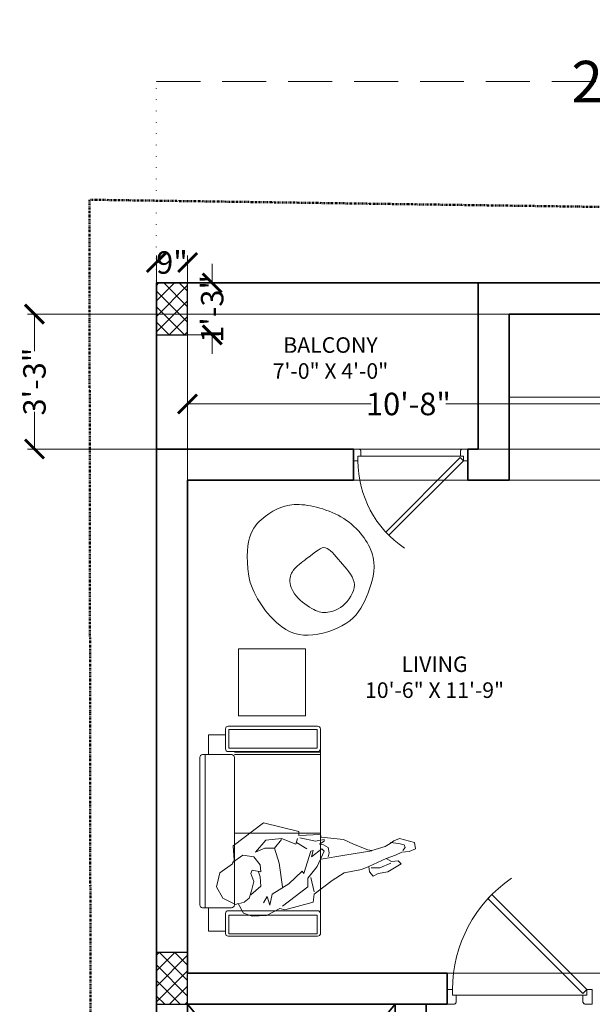
# Model space of a CAD drawing. Units: inches. Extents: x -16911 to -9621, y -48626 to -46270.
# Tile 13 of 20: x -12101 to -11935, y -46595 to -46311. Entities that reach past the tile are written whole.
import ezdxf

# ---------------------------------------------------------------- set-up
doc = ezdxf.new("R2010")
doc.units = ezdxf.units.IN
for name, pattern in [('DASHDOT', [1, 0.5, -0.25, 0, -0.25]), ('DASHED', [19.05, 12.7, -6.35]), ('DOT2', [3.175, 0, -3.175])]:
    doc.linetypes.add(name, pattern=pattern)
for name, color, linetype, lineweight in [('A-ANNO-DIMS', 2, 'Continuous', 13), ('A-AREA-IDEN', 3, 'Continuous', 18), ('A-DOOR', 4, 'Continuous', 18), ('A-FURN', 8, 'Continuous', 13), ('A-WALL', 7, 'Continuous', 35), ('C-PROP', 6, 'DASHDOT', 50), ('column', 12, 'Continuous', 30), ('DOOR', 143, 'Continuous', 9), ('EXT BEAM', 132, 'Continuous', 13), ('furniture', 35, 'Continuous', 15), ('Man', 8, 'Continuous', 5), ('S-BEAM', 132, 'Continuous', 25), ('S-COLS', 1, 'Continuous', 30)]:
    doc.layers.add(name, color=color, linetype=linetype, lineweight=lineweight)
doc.styles.add('style3', font='times.ttf')
doc.styles.add('style9', font='swisscl.ttf', dxfattribs={"height": 12})
doc.dimstyles.new('Dim9', dxfattribs={"dimtxt": 10, "dimasz": 0.199219, "dimexe": 1, "dimexo": 0.5, "dimgap": 1, "dimtad": 0, "dimdec": 1, "dimzin": 0, "dimdsep": 46, "dimlunit": 4, "dimtxsty": 'style9', "dimblk": 'ARCHTICK', "dimcen": 0.09, "dimclrd": 256, "dimclrt": 256, "dimadec": 0, "dimazin": 0, "dimtfac": 1, "dimtdec": 1, "dimtix": 1, "dimtofl": 0, "dimtmove": 1, "dimatfit": 3, "dimfxl": 9, "dimtolj": 1, "dimtzin": 0, "dimlwd": -1, "dimarcsym": 0})
doc.dimstyles.new('S.S.S', dxfattribs={"dimtxt": 6.5, "dimasz": 5.5, "dimexe": 2, "dimexo": 0, "dimgap": 0.09, "dimtad": 0, "dimdec": 1, "dimzin": 3, "dimdsep": 46, "dimlunit": 4, "dimtxsty": 'style3', "dimblk": 'ARCHTICK', "dimcen": 2.5, "dimclrd": 252, "dimclre": 256, "dimclrt": 7, "dimadec": 0, "dimazin": 0, "dimtfac": 1, "dimtdec": 1, "dimtix": 1, "dimtofl": 0, "dimtmove": 0, "dimatfit": 3, "dimfxl": 2, "dimtolj": 1, "dimtzin": 0, "dimlwd": 13, "dimlwe": 15, "dimarcsym": 0})

# ---------------------------------------------------------------- blocks, each defined once
blk = doc.blocks.new('Bipman02')
blk.add_lwpolyline([(0.5871, -0.067), (0.6175, -0.0496), (0.6523, -0.0539), (0.6697, -0.0376), (0.5958, 0.0069), (0.5437, 0.0156), (0.5164, 0.0297), (0.4959, 0.0069), (0.4915, -0.0235), (0.4524, -0.0061), (0.3568, 0.0113), (0.2917, 0.0548), (0.1917, 0.1287), (0.1874, 0.1722), (0.031, 0.2156), (0.0049, 0.2069), (-0.0689, 0.2461), (-0.1471, 0.2504), (-0.1949, 0.233), (-0.2253, 0.1808), (-0.2384, 0.1852), (-0.3079, 0.1504), (-0.3426, 0.0895), (-0.3253, 0.0113), (-0.2558, -0.0365), (-0.2471, -0.0583), (-0.2514, -0.1365), (-0.0863, -0.2626), (0.1092, -0.2148), (0.1092, -0.193), (0.2265, -0.1974), (0.2308, -0.1844), (0.3525, -0.1713), (0.409, -0.1452), (0.4872, -0.1148), (0.5089, -0.1104), (0.5828, -0.1322), (0.6088, -0.1496), (0.6295, -0.1636), (0.661, -0.1757), (0.7435, -0.1539), (0.7478, -0.1191), (0.7143, -0.1051), (0.674, -0.1017), (0.6392, -0.0844)], close=True)
for points in [[(-0.2558, -0.0452), (-0.1993, -0.0844), (-0.1385, -0.0757), (-0.1037, -0.0322), (-0.0994, 0.0069), (-0.1471, -0.0018), (-0.1558, 0.0156), (-0.1385, 0.0591), (-0.1515, 0.1113), (-0.1645, 0.1504), (-0.1906, 0.1722), (-0.2167, 0.1808)], [(-0.0863, 0.1765), (-0.0646, 0.1417), (-0.0516, 0.1895), (-0.0385, 0.1287), (0.0527, 0.0722), (0.1266, 0.0026), (0.1353, 0.0156), (0.1744, -0.1061), (0.1874, -0.1104), (0.1787, -0.0757), (0.2352, -0.1191), (0.2482, -0.1061), (0.2091, -0.0235), (0.157, 0.0417), (0.157, 0.0895), (0.018, 0.1939)], [(-0.1558, 0.133), (-0.0994, 0.0852), (-0.1037, 0.033), (-0.1124, 0.0069)], [(0.1917, 0.1156), (0.1744, 0.0374)], [(0.018, 0.0895), (0.0006, -0.0409), (-0.0255, -0.1235), (-0.0776, -0.1235), (-0.1298, -0.1017), (-0.0733, -0.167), (0.0136, -0.1757), (0.0918, -0.1452), (0.1005, -0.1757)], [(0.4915, -0.0235), (0.5871, -0.067)], [(0.5045, -0.0148), (0.5523, -0.0148), (0.6132, -0.0409)], [(0.2699, -0.0757), (0.2743, -0.0974), (0.2699, -0.1278), (0.2439, -0.1409), (0.2222, -0.1452), (0.2482, -0.1626), (0.2482, -0.1713), (0.2004, -0.1626), (0.1135, -0.18)], [(0.2308, -0.0626), (0.3612, -0.0844), (0.5089, -0.1095)], [(-0.0255, -0.1235), (0.0136, -0.1713)], [(0.0962, -0.1539), (0.1526, -0.1191)], [(0.6783, -0.1104), (0.6914, -0.1278), (0.687, -0.1409), (0.6566, -0.1496), (0.6088, -0.1539)]]:
    blk.add_lwpolyline(points)
blk = doc.blocks.new('erertety')
at = {"layer": 'furniture', "ltscale": 0.2}
for p, q in [((-17662.13, -45230.66), (-17662.13, -45176.69)), ((-17693.83, -45223.2), (-17693.83, -45184.43)), ((-17685.49, -45183.68), (-17693.08, -45183.68)), ((-17684.74, -45223.2), (-17684.74, -45184.43)), ((-17684.74, -45203.31), (-17662.13, -45203.31)), ((-17685.49, -45223.95), (-17693.08, -45223.95)), ((-17691.58, -45223.95), (-17691.58, -45229.1)), ((-17684.74, -45223.99), (-17662.13, -45223.99)), ((-17684.74, -45224.55), (-17662.13, -45224.55)), ((-17684.74, -45224.55), (-17662.13, -45224.55)), ((-17691.58, -45229.1), (-17687.09, -45229.1))]:
    blk.add_line(p, q, dxfattribs=at)
for points in [[(-17662.13, -45182.17), (-17662.13, -45176.97, 0.414214), (-17662.87, -45176.22), (-17686.34, -45176.22, 0.414214), (-17687.09, -45176.97), (-17687.09, -45182.17, 0.414214), (-17686.34, -45182.91), (-17662.87, -45182.91, 0.414214)], [(-17662.13, -45225.47), (-17662.13, -45230.66, -0.414214), (-17662.87, -45231.41), (-17686.34, -45231.41, -0.414214), (-17687.09, -45230.66), (-17687.09, -45225.47, -0.414214), (-17686.34, -45224.72), (-17662.87, -45224.72, -0.414214)]]:
    blk.add_lwpolyline(points, format="xyb", close=True, dxfattribs=at)
for points in [[(-17663.01, -45181.75), (-17663.01, -45176.82), (-17686.21, -45176.82), (-17686.21, -45181.75)], [(-17692.4, -45183.68), (-17692.4, -45223.95), (-17692.4, -45223.95), (-17692.4, -45183.68)], [(-17663.01, -45225.6), (-17663.01, -45230.53), (-17686.21, -45230.53), (-17686.21, -45225.6)]]:
    blk.add_lwpolyline(points, close=True, dxfattribs=at)
blk.add_lwpolyline([(-17687.09, -45177.54), (-17691.58, -45177.54), (-17691.58, -45183.68)], dxfattribs=at)
for centre, start, end in [((-17693.08, -45184.43), 90, 180), ((-17685.49, -45184.43), 0, 90), ((-17693.08, -45223.2), 180, 270), ((-17685.49, -45223.2), 270, 0)]:
    blk.add_arc(centre, 0.748, start, end, dxfattribs=at)
at = {"layer": 'furniture', "ltscale": 0.2, "xscale": 47.90818138957024, "yscale": 47.90818138957024, "zscale": 47.90818138957024}
blk.add_blockref('Bipman02', (-17673, -45193.44, 0), dxfattribs=at)
blk = doc.blocks.new('rthrty')
at = {"layer": 'furniture'}
blk.add_open_spline([(-17650.3, -45154.53), (-17651.97, -45142.9), (-17645.3, -45136.31), (-17637.11, -45132.37), (-17620.71, -45137.17), (-17612.47, -45149.45), (-17615.73, -45159.71), (-17619.67, -45168.02), (-17632.28, -45172.65), (-17641.84, -45170.43), (-17649.5, -45159.42), (-17650.3, -45154.53)], degree=3, dxfattribs=at)
at = {"layer": 'Man'}
blk.add_open_spline([(-17632.99, -45149.02), (-17629.89, -45146.6), (-17628, -45145.12), (-17623.29, -45151.15), (-17618.06, -45156.77), (-17623.15, -45164.08), (-17628.28, -45165.32), (-17631.61, -45164.6), (-17638.01, -45159.61), (-17638.81, -45154.69), (-17636.9, -45151.81), (-17632.99, -45149.02), (-17632.99, -45149.02)], degree=3, dxfattribs=at)
blk = doc.blocks.new('A$C1C9D3E54')
at = {"layer": 'DOOR'}
blk.add_line((18676.53, 5780.72), (18710.53, 5780.72), dxfattribs=at)
blk.add_lwpolyline([(18685.01, 5806.62), (18710.47, 5781.16), (18711.53, 5782.22), (18686.07, 5807.68), (18685.01, 5806.62)], dxfattribs=at)
blk.add_lwpolyline([(18674.03, 5778.22), (18676.03, 5778.22), (18674.03, 5778.22), (18674.03, 5782.22), (18675.53, 5782.22), (18675.53, 5780.72), (18676.53, 5780.72), (18676.53, 5778.72), (18676.41, 5778.72), (18676.41, 5778.6, -0.414214), (18676.16, 5778.35), (18676.03, 5778.35), (18676.03, 5778.22)], format="xyb", dxfattribs=at)
blk.add_lwpolyline([(18713.03, 5782.22), (18711.53, 5782.22), (18711.53, 5780.72), (18710.53, 5780.72), (18710.53, 5778.72), (18710.66, 5778.72), (18710.66, 5778.6, 0.414214), (18710.91, 5778.35), (18711.03, 5778.35), (18711.03, 5778.22), (18713.03, 5778.22), (18711.03, 5778.22), (18713.03, 5778.22), (18713.03, 5782.22)], format="xyb", close=True, dxfattribs=at)
blk.add_arc((18711.53, 5782.22), 36, 124.0336, 180, dxfattribs=at)
blk = doc.blocks.new('COLUMNS')
at = {"layer": 'column'}
h = blk.add_hatch(dxfattribs=at)
h.set_pattern_fill('ANSI37', color=256, angle=-720)
h.set_pattern_definition([(45, (21703.4588, -104481.6704), (-2.24506403, 2.24506403), []), (135, (21703.4588, -104481.6704), (-2.24506403, -2.24506403), [])])
h.paths.add_polyline_path([(-12061.47, -46401.86), (-12052.47, -46401.86), (-12052.47, -46386.86), (-12061.47, -46386.86)])
h = blk.add_hatch(dxfattribs=at)
h.set_pattern_fill('ANSI37', color=256, angle=-900)
h.set_pattern_definition([(225, (-45817.4075, 11499.4594), (2.24506403, -2.24506403), []), (315, (-45817.4075, 11499.4594), (2.24506403, 2.24506403), [])])
h.paths.add_polyline_path([(-12052.47, -46580.36), (-12061.47, -46580.36), (-12061.47, -46595.36), (-12052.47, -46595.36)])
at = {"layer": 'column', "ltscale": 0.05}
for points in [[(-12052.47, -46386.86), (-12061.47, -46386.86), (-12061.47, -46401.86), (-12052.47, -46401.86)], [(-12061.47, -46595.36), (-12052.47, -46595.36), (-12052.47, -46580.36), (-12061.47, -46580.36)]]:
    blk.add_lwpolyline(points, close=True, dxfattribs=at)
blk = doc.blocks.new('TYPICAL BEAMS G-2')
at = {"layer": 'EXT BEAM'}
for p, q in [((-12061.47, -47658.74), (-11738.92, -47658.74)), ((-12061.47, -48216.7), (-12061.47, -47658.74)), ((-12052.47, -47667.74), (-11924.72, -47667.74)), ((-12052.47, -47939.24), (-12052.47, -47667.74)), ((-12052.47, -47706.74), (-11924.72, -47706.74)), ((-12052.47, -47715.74), (-11924.72, -47715.74)), ((-12052.47, -47858.24), (-11924.72, -47858.24))]:
    blk.add_line(p, q, dxfattribs=at)
blk = doc.blocks.new('_ArchTick')
at = {"color": 0, "linetype": 'ByBlock', "const_width": 0.15}
blk.add_lwpolyline([(-0.5, -0.5), (0.5, 0.5)], dxfattribs=at)
blk = doc.blocks.new('*D44')
at = {"layer": 'A-ANNO-DIMS', "color": 0, "lineweight": 15, "transparency": 16777216}
for p, q in [((-12052.47, -46395.86), (-12098.73, -46395.86)), ((-12052.47, -46434.86), (-12098.73, -46434.86))]:
    blk.add_line(p, q, dxfattribs=at)
at = {"layer": 'A-ANNO-DIMS', "color": 0, "lineweight": 13, "transparency": 16777216}
for p, q in [((-12096.73, -46395.86), (-12096.73, -46406.56)), ((-12096.73, -46434.86), (-12096.73, -46424.15))]:
    blk.add_line(p, q, dxfattribs=at)
at = {"layer": 'Defpoints', "color": 0, "transparency": 16777216}
for p in [(-12052.47, -46395.86), (-12096.73, -46434.86), (-12052.47, -46434.86)]:
    blk.add_point(p, dxfattribs=at)
at = {"layer": 'A-ANNO-DIMS', "color": 0, "lineweight": 13, "transparency": 16777216, "xscale": 5.5, "yscale": 5.5, "zscale": 5.5}
for p, rotation in [((-12096.73, -46395.86), 90), ((-12096.73, -46434.86), 270)]:
    blk.add_blockref('_ArchTick', p, dxfattribs=dict(at, rotation=rotation))
at = {"layer": 'A-ANNO-DIMS', "color": 0, "transparency": 16777216, "insert": (-12096.73, -46415.36), "char_height": 6.5, "attachment_point": 5, "rotation": 90, "style": 'style3'}
blk.add_mtext('\\A1;3\'-3"', dxfattribs=at)
blk = doc.blocks.new('*D45')
at = {"layer": 'A-ANNO-DIMS', "color": 0, "lineweight": 15, "transparency": 16777216}
for p, q in [((-12052.47, -46434.86), (-12052.47, -46419.84)), ((-11924.72, -46434.86), (-11924.72, -46419.84))]:
    blk.add_line(p, q, dxfattribs=at)
at = {"layer": 'A-ANNO-DIMS', "color": 0, "lineweight": 13, "transparency": 16777216}
for p, q in [((-12052.47, -46421.84), (-11999.43, -46421.84)), ((-11924.72, -46421.84), (-11977.77, -46421.84))]:
    blk.add_line(p, q, dxfattribs=at)
at = {"layer": 'Defpoints', "color": 0, "transparency": 16777216}
for p in [(-11924.72, -46421.84), (-12052.47, -46434.86), (-11924.72, -46434.86)]:
    blk.add_point(p, dxfattribs=at)
at = {"layer": 'A-ANNO-DIMS', "color": 0, "lineweight": 13, "transparency": 16777216, "xscale": 5.5, "yscale": 5.5, "zscale": 5.5, "rotation": 180}
blk.add_blockref('_ArchTick', (-12052.47, -46421.84), dxfattribs=at)
at = {"layer": 'A-ANNO-DIMS', "color": 0, "lineweight": 13, "transparency": 16777216, "xscale": 5.5, "yscale": 5.5, "zscale": 5.5}
blk.add_blockref('_ArchTick', (-11924.72, -46421.84), dxfattribs=at)
at = {"layer": 'A-ANNO-DIMS', "color": 0, "transparency": 16777216, "insert": (-11988.6, -46421.84), "char_height": 6.5, "attachment_point": 5, "style": 'style3'}
blk.add_mtext('\\A1;10\'-8"', dxfattribs=at)
blk = doc.blocks.new('*D48')
at = {"layer": 'A-ANNO-DIMS', "color": 0, "lineweight": 15, "transparency": 16777216}
for p, q in [((-12061.47, -46386.86), (-12061.47, -46378.94)), ((-12052.47, -46386.86), (-12052.47, -46378.94))]:
    blk.add_line(p, q, dxfattribs=at)
at = {"layer": 'A-ANNO-DIMS', "color": 0, "lineweight": 13, "transparency": 16777216}
for p, q in [((-12061.47, -46380.94), (-12060.91, -46380.94)), ((-12052.47, -46380.94), (-12053.03, -46380.94))]:
    blk.add_line(p, q, dxfattribs=at)
at = {"layer": 'Defpoints', "color": 0, "transparency": 16777216}
for p in [(-12052.47, -46380.94), (-12061.47, -46386.86), (-12052.47, -46386.86)]:
    blk.add_point(p, dxfattribs=at)
at = {"layer": 'A-ANNO-DIMS', "color": 0, "lineweight": 13, "transparency": 16777216, "xscale": 5.5, "yscale": 5.5, "zscale": 5.5, "rotation": 180}
blk.add_blockref('_ArchTick', (-12061.47, -46380.94), dxfattribs=at)
at = {"layer": 'A-ANNO-DIMS', "color": 0, "lineweight": 13, "transparency": 16777216, "xscale": 5.5, "yscale": 5.5, "zscale": 5.5}
blk.add_blockref('_ArchTick', (-12052.47, -46380.94), dxfattribs=at)
at = {"layer": 'A-ANNO-DIMS', "color": 0, "transparency": 16777216, "insert": (-12056.97, -46380.94), "char_height": 6.5, "attachment_point": 5, "style": 'style3'}
blk.add_mtext('\\A1;9"', dxfattribs=at)
blk = doc.blocks.new('*D49')
at = {"layer": 'A-ANNO-DIMS', "color": 0, "lineweight": 13, "transparency": 16777216}
for p, q in [((-12045.35, -46386.86), (-12045.35, -46381.36)), ((-12045.35, -46401.86), (-12045.35, -46407.36))]:
    blk.add_line(p, q, dxfattribs=at)
at = {"layer": 'A-ANNO-DIMS', "color": 0, "lineweight": 15, "transparency": 16777216}
for p, q in [((-12052.47, -46386.86), (-12043.35, -46386.86)), ((-12052.47, -46401.86), (-12043.35, -46401.86))]:
    blk.add_line(p, q, dxfattribs=at)
at = {"layer": 'Defpoints', "color": 0, "transparency": 16777216}
for p in [(-12052.47, -46386.86), (-12052.47, -46401.86), (-12045.35, -46401.86)]:
    blk.add_point(p, dxfattribs=at)
at = {"layer": 'A-ANNO-DIMS', "color": 0, "lineweight": 13, "transparency": 16777216, "xscale": 5.5, "yscale": 5.5, "zscale": 5.5}
for p, rotation in [((-12045.35, -46386.86), 270), ((-12045.35, -46401.86), 90)]:
    blk.add_blockref('_ArchTick', p, dxfattribs=dict(at, rotation=rotation))
at = {"layer": 'A-ANNO-DIMS', "color": 0, "transparency": 16777216, "insert": (-12045.35, -46394.36), "char_height": 6.5, "attachment_point": 5, "rotation": 90, "style": 'style3'}
blk.add_mtext('\\A1;1\'-3"', dxfattribs=at)
blk = doc.blocks.new('*D114')
at = {"layer": 'A-ANNO-DIMS', "color": 0, "linetype": 'DOT2', "lineweight": -2, "transparency": 16777216}
for p, q in [((-12061.47, -46386.36), (-12061.47, -46327.66)), ((-11738.92, -46386.36), (-11738.92, -46327.66))]:
    blk.add_line(p, q, dxfattribs=at)
at = {"layer": 'A-ANNO-DIMS', "linetype": 'DASHED', "transparency": 16777216}
for p, q in [((-12061.47, -46328.66), (-11933.21, -46328.66)), ((-11738.92, -46328.66), (-11867.19, -46328.66))]:
    blk.add_line(p, q, dxfattribs=at)
at = {"layer": 'Defpoints', "color": 0, "transparency": 16777216}
for p in [(-11738.92, -46328.66), (-12061.47, -46386.86), (-11738.92, -46386.86)]:
    blk.add_point(p, dxfattribs=at)
at = {"layer": 'A-ANNO-DIMS', "transparency": 16777216, "xscale": 0.19921875, "yscale": 0.19921875, "zscale": 0.19921875, "rotation": 180}
blk.add_blockref('_ArchTick', (-12061.47, -46328.66), dxfattribs=at)
at = {"layer": 'A-ANNO-DIMS', "transparency": 16777216, "xscale": 0.19921875, "yscale": 0.19921875, "zscale": 0.19921875}
blk.add_blockref('_ArchTick', (-11738.92, -46328.66), dxfattribs=at)
at = {"layer": 'A-ANNO-DIMS', "transparency": 16777216, "insert": (-11900.2, -46328.66), "char_height": 12, "attachment_point": 5, "style": 'style9'}
blk.add_mtext('\\A1;26\'-10 1/2"', dxfattribs=at)

msp = doc.modelspace()

# ---------------------------------------------------------------- linework, layer by layer
at = {"layer": 'A-FURN', "ltscale": 0.2}
msp.add_line((-11795.925, -46419.855), (-11959.474, -46419.855), dxfattribs=at)
at = {"layer": 'A-FURN'}
msp.add_lwpolyline([(-12018.353, -46511.978), (-12037.713, -46511.978), (-12037.713, -46492.618), (-12018.353, -46492.618)], close=True, dxfattribs=at)
at = {"layer": 'A-WALL'}
for p, q in [((-12061.474, -46434.855), (-12061.474, -46386.855)), ((-11968.474, -46386.855), (-12061.474, -46386.855)), ((-11968.474, -46434.855), (-11968.474, -46386.855)), ((-11738.925, -46386.855), (-11968.474, -46386.855)), ((-11959.474, -46443.855), (-11959.474, -46395.855)), ((-11795.925, -46395.855), (-11959.474, -46395.855)), ((-12061.474, -46896.809), (-12061.474, -46434.855)), ((-12004.474, -46434.855), (-12061.474, -46434.855)), ((-12004.474, -46434.855), (-12004.474, -46443.855)), ((-11968.474, -46434.855), (-11971.474, -46434.855)), ((-11971.474, -46434.855), (-11971.474, -46443.855)), ((-12052.474, -46586.355), (-12052.474, -46443.855)), ((-12004.474, -46443.855), (-12052.474, -46443.855)), ((-11959.474, -46443.855), (-11971.474, -46443.855)), ((-11977.474, -46586.355), (-12052.474, -46586.355)), ((-11977.474, -46595.355), (-11977.474, -46586.355)), ((-12052.474, -46667.355), (-12052.474, -46595.355)), ((-11977.474, -46595.355), (-12052.474, -46595.355)), ((-12052.474, -46595.355), (-11992.474, -46667.355)), ((-12052.474, -46667.355), (-11992.474, -46595.355)), ((-11992.474, -46667.355), (-11992.474, -46595.355)), ((-11983.474, -46667.355), (-11983.474, -46595.355))]:
    msp.add_line(p, q, dxfattribs=at)
at = {"layer": 'C-PROP'}
msp.add_lwpolyline([(-12080.474, -46962.809), (-11720.293, -46969.035), (-11719.732, -46940.446), (-11720.395, -46855.606), (-11721.561, -46609.511), (-11721.175, -46367.855), (-12080.838, -46362.811), (-12080.3, -46762.955)], close=True, dxfattribs=at)

# ---------------------------------------------------------------- block references
at = {"layer": 'A-DOOR', "xscale": -0.8461538461538624, "yscale": 0.8461538461538624, "zscale": 0.8461538461538624, "rotation": 180}
msp.add_blockref('A$C1C9D3E54', (-27805.577, -41545.589), dxfattribs=at)
at = {"layer": 'A-DOOR', "xscale": 1.076923076922859, "yscale": 1.076923076922859, "zscale": 1.076923076922859}
msp.add_blockref('A$C1C9D3E54', (-32087.969, -52818.058), dxfattribs=at)
at = {"layer": 'A-FURN'}
msp.add_blockref('rthrty', (5615.537, -1317.075), dxfattribs=at)
at = {"layer": 'A-FURN', "xscale": -1.1, "yscale": 1.1, "zscale": 1.1, "rotation": 180}
msp.add_blockref('erertety', (7414.285, -96269.509, 0), dxfattribs=at)
at = {"layer": 'S-BEAM'}
msp.add_blockref('TYPICAL BEAMS G-2', (0, 1271.886), dxfattribs=at)
at = {"layer": 'S-COLS'}
msp.add_blockref('COLUMNS', (0, 0), dxfattribs=at)

# ---------------------------------------------------------------- texts
at = {"layer": 'A-AREA-IDEN', "ltscale": 10, "char_height": 4.5, "width": 42.823, "attachment_point": 1, "style": 'style9'}
for s, insert in [('\\A1;\\pxqc;{\\fCentury Gothic|b0|i0|c0|p34;BALCONY\\P7\'-0" X 4\'-0"}', (-12032.568, -46402.553)), ('\\A1;\\pxqc;{\\fCentury Gothic|b0|i0|c0|p34;LIVING\\P10\'-6" X 11\'-9"}', (-12002.486, -46494.801))]:
    msp.add_mtext(s, dxfattribs=dict(at, insert=insert))

# ---------------------------------------------------------------- dimensions: what is measured, and where the dimension line sits
at = {"layer": 'A-ANNO-DIMS'}
for base, p1, p2, dimstyle, override, picture, middle in [((-11738.925, -46328.661), (-12061.474, -46386.855), (-11738.925, -46386.855), 'Dim9', {"dimdec": 1, "dimlfac": 1, "dimrnd": 0, "dimzin": 1, "dimdsep": 46, "dimlunit": 4, "dimfrac": 2}, '*D114', (-11900.199, -46328.661)), ((-12052.474, -46380.945), (-12061.474, -46386.855), (-12052.474, -46386.855), 'S.S.S', {"dimclrd": 0, "dimclre": 0, "dimclrt": 0}, '*D48', (-12056.974, -46380.945)), ((-11924.724314023, -46421.841338665), (-12052.474314023, -46434.855496681), (-11924.724314023, -46434.855496681), 'S.S.S', {"dimclrd": 0, "dimclre": 0, "dimclrt": 0}, '*D45', (-11988.599314023, -46421.841338665))]:
    dim = msp.add_linear_dim(base=base, p1=p1, p2=p2, dimstyle=dimstyle, override=override, dxfattribs=at)
    dim.commit()
    dim.dimension.update_dxf_attribs({"geometry": picture, "text_midpoint": middle})
for base, p1, p2, picture, middle in [((-12045.346, -46401.855), (-12052.474, -46386.855), (-12052.474, -46401.855), '*D49', (-12045.346, -46394.355)), ((-12096.726, -46434.855), (-12052.474, -46395.855), (-12052.474, -46434.855), '*D44', (-12096.726, -46415.355))]:
    dim = msp.add_linear_dim(base=base, p1=p1, p2=p2, angle=90, dimstyle='S.S.S', override={"dimclrd": 0, "dimclre": 0, "dimclrt": 0}, dxfattribs=at)
    dim.commit()
    dim.dimension.update_dxf_attribs({"geometry": picture, "text_midpoint": middle})

doc.saveas('drawing.dxf')
